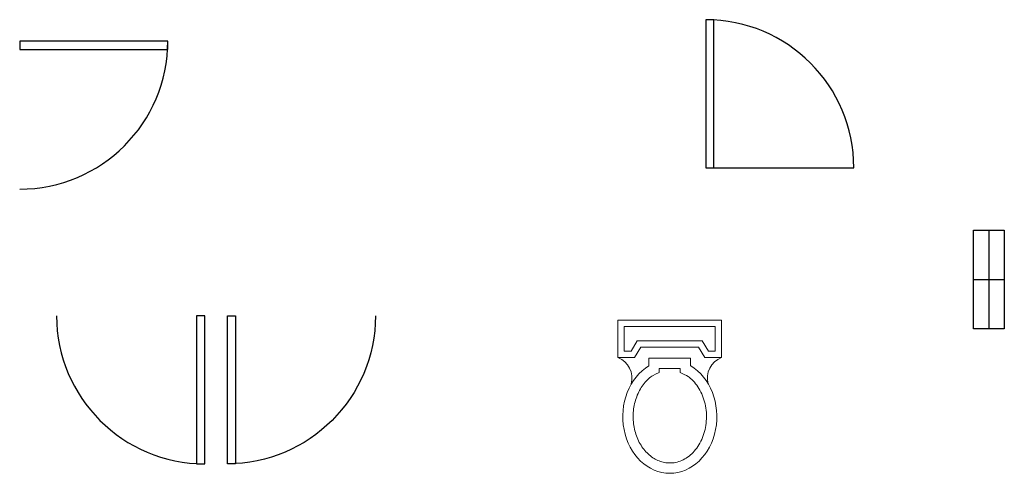
# Model space of a CAD drawing. Units: inches. Extents: x 604 to 3492, y -123 to 1737.
# Tile 20 of 20: x 3013 to 3492, y 647 to 868. Entities that reach past the tile are written whole.
import ezdxf

# ---------------------------------------------------------------- set-up
doc = ezdxf.new("R2010")
doc.units = ezdxf.units.IN
for name, color, linetype, lineweight in [('A-DOOR', 3, 'Continuous', 25), ('A-FLOR-FIXT', 9, 'Continuous', 18), ('A-GLAZ', 4, 'Continuous', 25)]:
    doc.layers.add(name, color=color, linetype=linetype, lineweight=lineweight)

# ---------------------------------------------------------------- blocks, each defined once
blk = doc.blocks.new('A$C7C8779AE')
for p, q in [((0, 0.7405), (0, 0.5605)), ((0.5, 0.7405), (0, 0.7405)), ((0.5, 0.5605), (0.5, 0.7405)), ((0.47, 0.7105), (0.03, 0.7105)), ((0.03, 0.7105), (0.03, 0.5905)), ((0.47, 0.5905), (0.47, 0.7105)), ((0.093, 0.6405), (0.063, 0.5905)), ((0.093, 0.6405), (0.407, 0.6405)), ((0.437, 0.5905), (0.407, 0.6405)), ((0.03, 0.5905), (0.063, 0.5905)), ((0.11, 0.6105), (0.08, 0.5605)), ((0.11, 0.6105), (0.39, 0.6105)), ((0.42, 0.5605), (0.39, 0.6105)), ((0.437, 0.5905), (0.47, 0.5905)), ((0, 0.5605), (0.08, 0.5605)), ((0.1497, 0.557), (0.1497, 0.5203)), ((0.1497, 0.557), (0.3514, 0.557)), ((0.3514, 0.557), (0.3514, 0.5203)), ((0.42, 0.5605), (0.5, 0.5605)), ((0.1997, 0.507), (0.1997, 0.4879)), ((0.1997, 0.507), (0.3014, 0.507)), ((0.3014, 0.507), (0.3014, 0.4879))]:
    blk.add_line(p, q)
for centre, start, end in [((-0.0386, 0.4613), 344.642, 68.7339), ((0.5386, 0.4613), 111.2661, 195.358)]:
    blk.add_arc(centre, 0.1064, start, end)
blk.add_ellipse((0.2506, 0.2744), major_axis=(0, 0.2744), ratio=0.828948, start_param=0.459479, end_param=5.823706)
blk.add_open_spline([(0.1997, 0.4879), (0.1697, 0.474), (0.1642, 0.4702), (0.1512, 0.4602), (0.1438, 0.4535), (0.1298, 0.4388), (0.1233, 0.4306), (0.1111, 0.4131), (0.1055, 0.4037), (0.0956, 0.3838), (0.0912, 0.3733), (0.0838, 0.3516), (0.0808, 0.3403), (0.0762, 0.3172), (0.0746, 0.3055), (0.073, 0.2817), (0.0729, 0.2698), (0.0743, 0.246), (0.0758, 0.2342), (0.0801, 0.2111), (0.0831, 0.1998), (0.0903, 0.1779), (0.0945, 0.1673), (0.1043, 0.1473), (0.1098, 0.1378), (0.1218, 0.12), (0.1283, 0.1118), (0.1421, 0.0968), (0.1494, 0.09), (0.1646, 0.078), (0.1725, 0.0728), (0.1887, 0.064), (0.1969, 0.0603), (0.2137, 0.0547), (0.2222, 0.0527), (0.2392, 0.0502), (0.2478, 0.0498), (0.2664, 0.0505), (0.2764, 0.052), (0.2963, 0.0573), (0.3061, 0.061), (0.3253, 0.0707), (0.3346, 0.0766), (0.3525, 0.0906), (0.3611, 0.0987), (0.3771, 0.1169), (0.3845, 0.127), (0.3978, 0.1488), (0.4037, 0.1605), (0.4137, 0.1853), (0.4178, 0.1983), (0.424, 0.2251), (0.4261, 0.2389), (0.4282, 0.2668), (0.4283, 0.2809), (0.4262, 0.3088), (0.4241, 0.3226), (0.418, 0.3495), (0.414, 0.3625), (0.404, 0.3873), (0.3982, 0.3991), (0.385, 0.421), (0.3776, 0.4311), (0.3617, 0.4494), (0.3531, 0.4575), (0.3382, 0.4693), (0.3321, 0.4736), (0.3014, 0.4879)], degree=3, knots=[0.459479, 0.459479, 0.459479, 0.459479, 0.567422, 0.567422, 0.720865, 0.720865, 0.874307, 0.874307, 1.02775, 1.02775, 1.181192, 1.181192, 1.334635, 1.334635, 1.488077, 1.488077, 1.64152, 1.64152, 1.794963, 1.794963, 1.948405, 1.948405, 2.101848, 2.101848, 2.25529, 2.25529, 2.408733, 2.408733, 2.562175, 2.562175, 2.715618, 2.715618, 2.86906, 2.86906, 3.022503, 3.022503, 3.175946, 3.175946, 3.356457, 3.356457, 3.536968, 3.536968, 3.717479, 3.717479, 3.89799, 3.89799, 4.078501, 4.078501, 4.259012, 4.259012, 4.439523, 4.439523, 4.620035, 4.620035, 4.800546, 4.800546, 4.981057, 4.981057, 5.161568, 5.161568, 5.342079, 5.342079, 5.52259, 5.52259, 5.703101, 5.703101, 5.823706, 5.823706, 5.823706, 5.823706])
blk = doc.blocks.new('DOOR-SWING-72')
for p, q in [((0, 72), (0, 0)), ((0, 0), (4, 0)), ((0, 0), (4, 0))]:
    blk.add_line(p, q)
blk.add_lwpolyline([(0, 72), (0, 0), (4, 0), (4, 72)], close=True)
blk.add_arc((0, 0), 72, 0, 90)
blk = doc.blocks.new('WIN-48')
for p, q in [((0, 48), (15, 48)), ((7.5, 48), (7.5, 0)), ((15, 48), (15, 0)), ((0, 24), (15, 24))]:
    blk.add_line(p, q)
blk.add_lwpolyline([(15, 0), (0, 0), (0, 48), (15, 48)], close=True)

msp = doc.modelspace()

# ---------------------------------------------------------------- linework, layer by layer
at = {"layer": 'A-DOOR'}
for p, q in [((3346.5764, 867.8269), (3346.5764, 795.8269)), ((3346.5764, 795.8269), (3350.5764, 795.8269)), ((3346.5764, 795.8269), (3418.5764, 795.8269))]:
    msp.add_line(p, q, dxfattribs=at)
msp.add_lwpolyline([(3346.5764, 867.8269), (3346.5764, 795.8269), (3350.5764, 795.8269), (3350.5764, 867.8269)], close=True, dxfattribs=at)
msp.add_arc((3346.5764, 795.8269), 72, 0, 90, dxfattribs=at)

# ---------------------------------------------------------------- block references
for p, rotation in [((3013.1261, 857.394), 269.9999999999998), ((3103.05, 723.8269), 180)]:
    msp.add_blockref('DOOR-SWING-72', p, dxfattribs=dict(at, rotation=rotation))
at = {"layer": 'A-DOOR', "extrusion": (0, 0, -1), "zscale": -1, "rotation": 180}
msp.add_blockref('DOOR-SWING-72', (-3114.0679, 723.8269), dxfattribs=at)
at = {"layer": 'A-FLOR-FIXT', "xscale": 100.5290996938904, "yscale": 100.5290996938904, "zscale": 100.5290996938904}
msp.add_blockref('A$C7C8779AE', (3303.9537, 647.1866), dxfattribs=at)
at = {"layer": 'A-GLAZ'}
msp.add_blockref('WIN-48', (3476.7448, 717.4907), dxfattribs=at)

doc.saveas('drawing.dxf')
